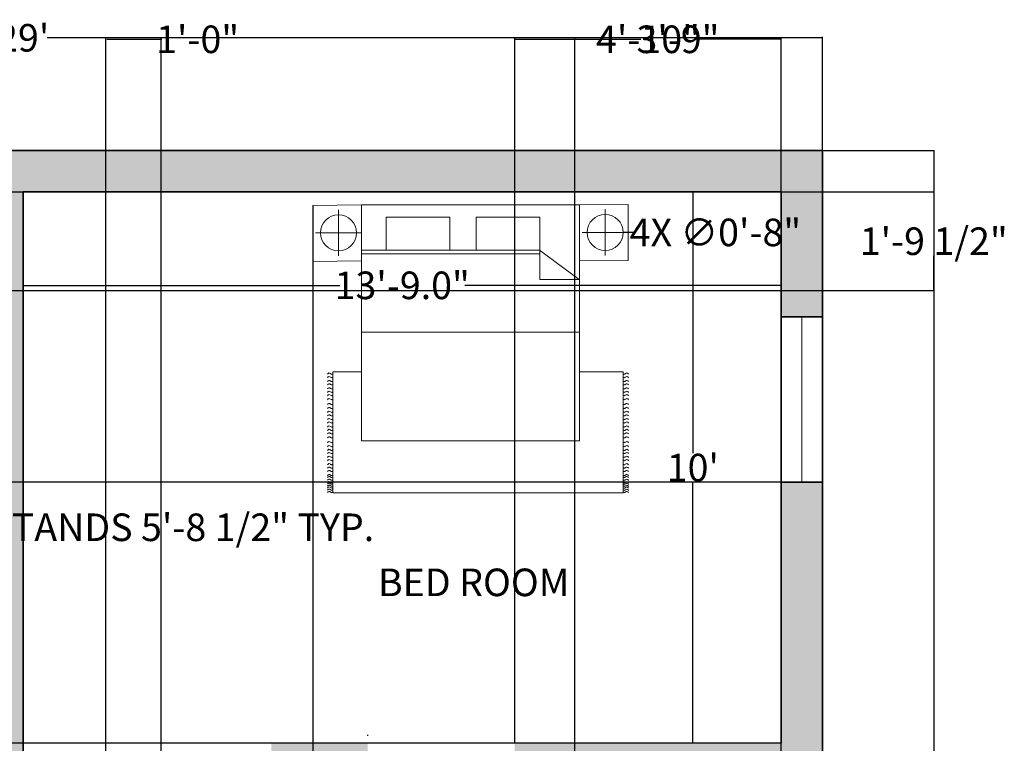
# Model space of a CAD drawing. Units: inches. Extents: x 1174 to 1615, y 3112 to 3628.
# Tile 6 of 6: x 1390 to 1604, y 3466 to 3623. Entities that reach past the tile are written whole.
import ezdxf

# ---------------------------------------------------------------- set-up
doc = ezdxf.new("R2010")
doc.units = ezdxf.units.IN
doc.header["$MEASUREMENT"] = 0
doc.layers.get('0').update_dxf_attribs({"color": 250})
for name, color, linetype, lineweight in [('A-ANNO-DIMS', 2, 'Continuous', 18), ('A-AREA-IDEN', 7, 'Continuous', 25), ('A-FURN', 8, 'Continuous', 13), ('A-GLAZ', 4, 'Continuous', 18), ('A-WALL', 7, 'Continuous', 35)]:
    doc.layers.add(name, color=color, linetype=linetype, lineweight=lineweight)
doc.layers.add('A-WALL-PATT', color=18, linetype='Continuous', lineweight=13, true_color=0x000000)
doc.styles.get("Standard").update_dxf_attribs({"font": 'arial.ttf'})
doc.dimstyles.get("Standard").update_dxf_attribs({"dimtxt": 6, "dimasz": 0.18, "dimexe": 0.18, "dimexo": 0.0625, "dimgap": 0.09, "dimtad": 0, "dimtih": 1, "dimtoh": 1, "dimdec": 1, "dimzin": 0, "dimdsep": 46, "dimlunit": 3, "dimtxsty": 'Standard', "dimcen": 0.09, "dimadec": 0, "dimazin": 0, "dimtfac": 1, "dimtdec": 1, "dimtofl": 0, "dimtmove": 0, "dimatfit": 3, "dimfxl": 1, "dimtolj": 1, "dimtzin": 0, "dimarcsym": 0})

# ---------------------------------------------------------------- blocks, each defined once
blk = doc.blocks.new('*D3')
at = {"layer": 'A-ANNO-DIMS', "color": 0, "lineweight": -2, "transparency": 16777216}
for p, q in [((1216.66, 3595.09), (1216.66, 3619.74)), ((1216.84, 3619.56), (1385.43, 3619.56)), ((1564.48, 3619.56), (1395.9, 3619.56)), ((1564.66, 3595.09), (1564.66, 3619.74))]:
    blk.add_line(p, q, dxfattribs=at)
at = {"layer": 'A-ANNO-DIMS', "color": 0, "transparency": 16777216}
for points in [[(1216.84, 3619.59), (1216.84, 3619.53), (1216.66, 3619.56)], [(1564.48, 3619.59), (1564.48, 3619.53), (1564.66, 3619.56)]]:
    blk.add_solid(points, dxfattribs=at)
at = {"layer": 'Defpoints', "color": 0, "transparency": 16777216}
for p in [(1564.66, 3619.56), (1216.66, 3595.03), (1564.66, 3595.03)]:
    blk.add_point(p, dxfattribs=at)
at = {"layer": 'A-ANNO-DIMS', "color": 0, "transparency": 16777216, "insert": (1390.66, 3619.56), "char_height": 6, "attachment_point": 5}
blk.add_mtext("\\A1;29'", dxfattribs=at)
blk = doc.blocks.new('*D15')
at = {"layer": 'A-ANNO-DIMS', "color": 0, "lineweight": -2, "transparency": 16777216}
for p, q in [((1555.6, 3586.03), (1536.24, 3586.03)), ((1536.42, 3585.85), (1536.42, 3529.18)), ((1536.42, 3466.21), (1536.42, 3522.88)), ((1555.6, 3466.03), (1536.24, 3466.03))]:
    blk.add_line(p, q, dxfattribs=at)
at = {"layer": 'A-ANNO-DIMS', "color": 0, "transparency": 16777216}
for points in [[(1536.39, 3585.85), (1536.45, 3585.85), (1536.42, 3586.03)], [(1536.39, 3466.21), (1536.45, 3466.21), (1536.42, 3466.03)]]:
    blk.add_solid(points, dxfattribs=at)
at = {"layer": 'Defpoints', "color": 0, "transparency": 16777216}
for p in [(1555.66, 3586.03), (1536.42, 3466.03), (1555.66, 3466.03)]:
    blk.add_point(p, dxfattribs=at)
at = {"layer": 'A-ANNO-DIMS', "color": 0, "transparency": 16777216, "insert": (1536.42, 3526.03), "char_height": 6, "attachment_point": 5}
blk.add_mtext("\\A1;10'", dxfattribs=at)
blk = doc.blocks.new('*D16')
at = {"layer": 'A-ANNO-DIMS', "color": 0, "lineweight": -2, "transparency": 16777216}
for p, q in [((1390.66, 3585.97), (1390.66, 3565.51)), ((1555.66, 3585.97), (1555.66, 3565.51)), ((1390.84, 3565.69), (1459.55, 3565.69)), ((1555.48, 3565.69), (1486.77, 3565.69))]:
    blk.add_line(p, q, dxfattribs=at)
at = {"layer": 'A-ANNO-DIMS', "color": 0, "transparency": 16777216}
for points in [[(1390.84, 3565.72), (1390.84, 3565.66), (1390.66, 3565.69)], [(1555.48, 3565.72), (1555.48, 3565.66), (1555.66, 3565.69)]]:
    blk.add_solid(points, dxfattribs=at)
at = {"layer": 'Defpoints', "color": 0, "transparency": 16777216}
for p in [(1390.66, 3586.03), (1555.66, 3586.03), (1555.66, 3565.69)]:
    blk.add_point(p, dxfattribs=at)
at = {"layer": 'A-ANNO-DIMS', "color": 0, "transparency": 16777216, "insert": (1473.16, 3565.69), "char_height": 6, "attachment_point": 5}
blk.add_mtext('\\A1;13\'-9.0"', dxfattribs=at)
blk = doc.blocks.new('BED-DOUBLE-WITH-NIGHTSTANDS')
for p, q in [((5.6, 61.61), (5.6, 51.56)), ((63.65, 61.72), (63.65, 51.66)), ((10.63, 56.59), (0.57, 56.59)), ((68.68, 56.69), (58.62, 56.69)), ((49.39, 52.82), (10.63, 52.82)), ((49.44, 52), (10.63, 52)), ((49.39, 52.82), (58, 46.47)), ((49.44, 52.82), (49.44, 46.47)), ((49.44, 46.47), (58, 46.47)), ((58.05, 34.96), (10.63, 34.96)), ((4.35, 0), (4.35, 26.37)), ((4.35, 26.37), (10.65, 26.37)), ((58.05, 26.37), (67.59, 26.37)), ((67.59, 26.37), (67.59, 0)), ((67.59, 0), (4.35, 0))]:
    blk.add_line(p, q)
for points in [[(0, 50.39), (10.63, 50.5), (10.63, 62.68), (0, 62.58)], [(58.05, 62.68), (58.05, 11.36), (10.63, 11.36), (10.63, 62.68)], [(58.05, 50.5), (68.68, 50.6), (68.68, 62.78), (58.05, 62.68)], [(29.88, 59.98), (29.88, 52.82), (15.98, 52.82), (15.98, 59.98)], [(49.44, 59.98), (49.44, 52.82), (35.55, 52.82), (35.55, 59.98)]]:
    blk.add_lwpolyline(points, close=True)
for centre in [(5.6, 56.59), (63.65, 56.69)]:
    blk.add_circle(centre, 3.92)
for points, knots in [([(3.23, 25.83), (3.32, 25.96), (3.52, 26.2), (3.86, 25.96), (4.14, 25.78), (4.29, 25.89), (4.35, 25.94)], [0, 0, 0, 0, 0.400747, 0.791423, 1.067667, 1.29709, 1.29709, 1.29709, 1.29709]), ([(68.71, 25.83), (68.61, 25.96), (68.42, 26.2), (68.08, 25.96), (67.8, 25.78), (67.65, 25.89), (67.58, 25.94)], [0, 0, 0, 0, 0.400747, 0.791423, 1.067667, 1.29709, 1.29709, 1.29709, 1.29709]), ([(3.23, 25.06), (3.32, 25.18), (3.52, 25.42), (3.86, 25.18), (4.14, 25.01), (4.29, 25.11), (4.35, 25.16)], [0, 0, 0, 0, 0.400747, 0.791423, 1.067667, 1.29709, 1.29709, 1.29709, 1.29709]), ([(3.23, 24.24), (3.32, 24.36), (3.52, 24.6), (3.86, 24.36), (4.14, 24.19), (4.29, 24.3), (4.35, 24.34)], [0, 0, 0, 0, 0.400747, 0.791423, 1.067667, 1.29709, 1.29709, 1.29709, 1.29709]), ([(3.23, 23.51), (3.32, 23.63), (3.52, 23.87), (3.86, 23.63), (4.14, 23.46), (4.29, 23.57), (4.35, 23.62)], [0, 0, 0, 0, 0.400747, 0.791423, 1.067667, 1.29709, 1.29709, 1.29709, 1.29709]), ([(68.71, 25.06), (68.61, 25.18), (68.42, 25.42), (68.08, 25.18), (67.8, 25.01), (67.65, 25.11), (67.58, 25.16)], [0, 0, 0, 0, 0.400747, 0.791423, 1.067667, 1.29709, 1.29709, 1.29709, 1.29709]), ([(68.71, 24.24), (68.61, 24.36), (68.42, 24.6), (68.08, 24.36), (67.8, 24.19), (67.65, 24.3), (67.58, 24.34)], [0, 0, 0, 0, 0.400747, 0.791423, 1.067667, 1.29709, 1.29709, 1.29709, 1.29709]), ([(68.71, 23.51), (68.61, 23.63), (68.42, 23.87), (68.08, 23.63), (67.8, 23.46), (67.65, 23.57), (67.58, 23.62)], [0, 0, 0, 0, 0.400747, 0.791423, 1.067667, 1.29709, 1.29709, 1.29709, 1.29709]), ([(3.23, 22.63), (3.32, 22.75), (3.52, 22.99), (3.86, 22.75), (4.14, 22.58), (4.29, 22.69), (4.35, 22.73)], [0, 0, 0, 0, 0.400747, 0.791423, 1.067667, 1.29709, 1.29709, 1.29709, 1.29709]), ([(3.23, 21.88), (3.32, 22), (3.52, 22.24), (3.86, 22), (4.14, 21.83), (4.29, 21.93), (4.35, 21.98)], [0, 0, 0, 0, 0.400747, 0.791423, 1.067667, 1.29709, 1.29709, 1.29709, 1.29709]), ([(68.71, 22.63), (68.61, 22.75), (68.42, 22.99), (68.08, 22.75), (67.8, 22.58), (67.65, 22.69), (67.58, 22.73)], [0, 0, 0, 0, 0.400747, 0.791423, 1.067667, 1.29709, 1.29709, 1.29709, 1.29709]), ([(68.71, 21.88), (68.61, 22), (68.42, 22.24), (68.08, 22), (67.8, 21.83), (67.65, 21.93), (67.58, 21.98)], [0, 0, 0, 0, 0.400747, 0.791423, 1.067667, 1.29709, 1.29709, 1.29709, 1.29709]), ([(3.23, 21.15), (3.32, 21.27), (3.52, 21.51), (3.86, 21.27), (4.14, 21.1), (4.29, 21.21), (4.35, 21.25)], [0, 0, 0, 0, 0.400747, 0.791423, 1.067667, 1.29709, 1.29709, 1.29709, 1.29709]), ([(3.23, 20.27), (3.32, 20.39), (3.52, 20.63), (3.86, 20.39), (4.14, 20.22), (4.29, 20.32), (4.35, 20.37)], [0, 0, 0, 0, 0.400747, 0.791423, 1.067667, 1.29709, 1.29709, 1.29709, 1.29709]), ([(3.23, 19.23), (3.32, 19.35), (3.52, 19.59), (3.86, 19.35), (4.14, 19.18), (4.29, 19.29), (4.35, 19.33)], [0, 0, 0, 0, 0.400747, 0.791423, 1.067667, 1.29709, 1.29709, 1.29709, 1.29709]), ([(68.71, 21.15), (68.61, 21.27), (68.42, 21.51), (68.08, 21.27), (67.8, 21.1), (67.65, 21.21), (67.58, 21.25)], [0, 0, 0, 0, 0.400747, 0.791423, 1.067667, 1.29709, 1.29709, 1.29709, 1.29709]), ([(68.71, 20.27), (68.61, 20.39), (68.42, 20.63), (68.08, 20.39), (67.8, 20.22), (67.65, 20.32), (67.58, 20.37)], [0, 0, 0, 0, 0.400747, 0.791423, 1.067667, 1.29709, 1.29709, 1.29709, 1.29709]), ([(68.71, 19.23), (68.61, 19.35), (68.42, 19.59), (68.08, 19.35), (67.8, 19.18), (67.65, 19.29), (67.58, 19.33)], [0, 0, 0, 0, 0.400747, 0.791423, 1.067667, 1.29709, 1.29709, 1.29709, 1.29709]), ([(3.23, 18.35), (3.32, 18.47), (3.52, 18.71), (3.86, 18.47), (4.14, 18.3), (4.29, 18.4), (4.35, 18.45)], [0, 0, 0, 0, 0.400747, 0.791423, 1.067667, 1.29709, 1.29709, 1.29709, 1.29709]), ([(3.23, 17.53), (3.32, 17.65), (3.52, 17.89), (3.86, 17.65), (4.14, 17.48), (4.29, 17.59), (4.35, 17.64)], [0, 0, 0, 0, 0.400747, 0.791423, 1.067667, 1.29709, 1.29709, 1.29709, 1.29709]), ([(68.71, 18.35), (68.61, 18.47), (68.42, 18.71), (68.08, 18.47), (67.8, 18.3), (67.65, 18.4), (67.58, 18.45)], [0, 0, 0, 0, 0.400747, 0.791423, 1.067667, 1.29709, 1.29709, 1.29709, 1.29709]), ([(68.71, 17.53), (68.61, 17.65), (68.42, 17.89), (68.08, 17.65), (67.8, 17.48), (67.65, 17.59), (67.58, 17.64)], [0, 0, 0, 0, 0.400747, 0.791423, 1.067667, 1.29709, 1.29709, 1.29709, 1.29709]), ([(3.23, 16.76), (3.32, 16.88), (3.52, 17.12), (3.86, 16.88), (4.14, 16.7), (4.29, 16.81), (4.35, 16.86)], [0, 0, 0, 0, 0.400747, 0.791423, 1.067667, 1.29709, 1.29709, 1.29709, 1.29709]), ([(3.23, 15.94), (3.32, 16.06), (3.52, 16.3), (3.86, 16.06), (4.14, 15.89), (4.29, 15.99), (4.35, 16.04)], [0, 0, 0, 0, 0.400747, 0.791423, 1.067667, 1.29709, 1.29709, 1.29709, 1.29709]), ([(3.23, 15.21), (3.32, 15.33), (3.52, 15.57), (3.86, 15.33), (4.14, 15.16), (4.29, 15.27), (4.35, 15.32)], [0, 0, 0, 0, 0.400747, 0.791423, 1.067667, 1.29709, 1.29709, 1.29709, 1.29709]), ([(68.71, 16.76), (68.61, 16.88), (68.42, 17.12), (68.08, 16.88), (67.8, 16.7), (67.65, 16.81), (67.58, 16.86)], [0, 0, 0, 0, 0.400747, 0.791423, 1.067667, 1.29709, 1.29709, 1.29709, 1.29709]), ([(68.71, 15.94), (68.61, 16.06), (68.42, 16.3), (68.08, 16.06), (67.8, 15.89), (67.65, 15.99), (67.58, 16.04)], [0, 0, 0, 0, 0.400747, 0.791423, 1.067667, 1.29709, 1.29709, 1.29709, 1.29709]), ([(68.71, 15.21), (68.61, 15.33), (68.42, 15.57), (68.08, 15.33), (67.8, 15.16), (67.65, 15.27), (67.58, 15.32)], [0, 0, 0, 0, 0.400747, 0.791423, 1.067667, 1.29709, 1.29709, 1.29709, 1.29709]), ([(3.23, 14.33), (3.32, 14.45), (3.52, 14.69), (3.86, 14.45), (4.14, 14.28), (4.29, 14.38), (4.35, 14.43)], [0, 0, 0, 0, 0.400747, 0.791423, 1.067667, 1.29709, 1.29709, 1.29709, 1.29709]), ([(3.23, 13.58), (3.32, 13.7), (3.52, 13.94), (3.86, 13.7), (4.14, 13.53), (4.29, 13.63), (4.35, 13.68)], [0, 0, 0, 0, 0.400747, 0.791423, 1.067667, 1.29709, 1.29709, 1.29709, 1.29709]), ([(3.23, 12.85), (3.32, 12.97), (3.52, 13.21), (3.86, 12.97), (4.14, 12.8), (4.29, 12.9), (4.35, 12.95)], [0, 0, 0, 0, 0.400747, 0.791423, 1.067667, 1.29709, 1.29709, 1.29709, 1.29709]), ([(68.71, 14.33), (68.61, 14.45), (68.42, 14.69), (68.08, 14.45), (67.8, 14.28), (67.65, 14.38), (67.58, 14.43)], [0, 0, 0, 0, 0.400747, 0.791423, 1.067667, 1.29709, 1.29709, 1.29709, 1.29709]), ([(68.71, 13.58), (68.61, 13.7), (68.42, 13.94), (68.08, 13.7), (67.8, 13.53), (67.65, 13.63), (67.58, 13.68)], [0, 0, 0, 0, 0.400747, 0.791423, 1.067667, 1.29709, 1.29709, 1.29709, 1.29709]), ([(68.71, 12.85), (68.61, 12.97), (68.42, 13.21), (68.08, 12.97), (67.8, 12.8), (67.65, 12.9), (67.58, 12.95)], [0, 0, 0, 0, 0.400747, 0.791423, 1.067667, 1.29709, 1.29709, 1.29709, 1.29709]), ([(3.23, 11.97), (3.32, 12.09), (3.52, 12.33), (3.86, 12.09), (4.14, 11.92), (4.29, 12.02), (4.35, 12.07)], [0, 0, 0, 0, 0.400747, 0.791423, 1.067667, 1.29709, 1.29709, 1.29709, 1.29709]), ([(3.23, 10.93), (3.32, 11.05), (3.52, 11.29), (3.86, 11.05), (4.14, 10.88), (4.29, 10.99), (4.35, 11.03)], [0, 0, 0, 0, 0.400747, 0.791423, 1.067667, 1.29709, 1.29709, 1.29709, 1.29709]), ([(68.71, 11.97), (68.61, 12.09), (68.42, 12.33), (68.08, 12.09), (67.8, 11.92), (67.65, 12.02), (67.58, 12.07)], [0, 0, 0, 0, 0.400747, 0.791423, 1.067667, 1.29709, 1.29709, 1.29709, 1.29709]), ([(68.71, 10.93), (68.61, 11.05), (68.42, 11.29), (68.08, 11.05), (67.8, 10.88), (67.65, 10.99), (67.58, 11.03)], [0, 0, 0, 0, 0.400747, 0.791423, 1.067667, 1.29709, 1.29709, 1.29709, 1.29709]), ([(3.23, 10.05), (3.32, 10.17), (3.52, 10.41), (3.86, 10.17), (4.14, 10), (4.29, 10.1), (4.35, 10.15)], [0, 0, 0, 0, 0.400747, 0.791423, 1.067667, 1.29709, 1.29709, 1.29709, 1.29709]), ([(3.23, 9.23), (3.32, 9.35), (3.52, 9.59), (3.86, 9.35), (4.14, 9.18), (4.29, 9.29), (4.35, 9.34)], [0, 0, 0, 0, 0.400747, 0.791423, 1.067667, 1.29709, 1.29709, 1.29709, 1.29709]), ([(3.23, 8.54), (3.32, 8.66), (3.52, 8.9), (3.86, 8.66), (4.14, 8.49), (4.29, 8.6), (4.35, 8.65)], [0, 0, 0, 0, 0.400747, 0.791423, 1.067667, 1.29709, 1.29709, 1.29709, 1.29709]), ([(68.71, 10.05), (68.61, 10.17), (68.42, 10.41), (68.08, 10.17), (67.8, 10), (67.65, 10.1), (67.58, 10.15)], [0, 0, 0, 0, 0.400747, 0.791423, 1.067667, 1.29709, 1.29709, 1.29709, 1.29709]), ([(68.71, 9.23), (68.61, 9.35), (68.42, 9.59), (68.08, 9.35), (67.8, 9.18), (67.65, 9.29), (67.58, 9.34)], [0, 0, 0, 0, 0.400747, 0.791423, 1.067667, 1.29709, 1.29709, 1.29709, 1.29709]), ([(68.71, 8.54), (68.61, 8.66), (68.42, 8.9), (68.08, 8.66), (67.8, 8.49), (67.65, 8.6), (67.58, 8.65)], [0, 0, 0, 0, 0.400747, 0.791423, 1.067667, 1.29709, 1.29709, 1.29709, 1.29709]), ([(3.23, 7.73), (3.32, 7.85), (3.52, 8.09), (3.86, 7.85), (4.14, 7.68), (4.29, 7.78), (4.35, 7.83)], [0, 0, 0, 0, 0.400747, 0.791423, 1.067667, 1.29709, 1.29709, 1.29709, 1.29709]), ([(3.23, 7), (3.32, 7.12), (3.52, 7.36), (3.86, 7.12), (4.14, 6.95), (4.29, 7.05), (4.35, 7.1)], [0, 0, 0, 0, 0.400747, 0.791423, 1.067667, 1.29709, 1.29709, 1.29709, 1.29709]), ([(68.71, 7.73), (68.61, 7.85), (68.42, 8.09), (68.08, 7.85), (67.8, 7.68), (67.65, 7.78), (67.58, 7.83)], [0, 0, 0, 0, 0.400747, 0.791423, 1.067667, 1.29709, 1.29709, 1.29709, 1.29709]), ([(68.71, 7), (68.61, 7.12), (68.42, 7.36), (68.08, 7.12), (67.8, 6.95), (67.65, 7.05), (67.58, 7.1)], [0, 0, 0, 0, 0.400747, 0.791423, 1.067667, 1.29709, 1.29709, 1.29709, 1.29709]), ([(3.23, 6.12), (3.32, 6.24), (3.52, 6.48), (3.86, 6.24), (4.14, 6.06), (4.29, 6.17), (4.35, 6.22)], [0, 0, 0, 0, 0.400747, 0.791423, 1.067667, 1.29709, 1.29709, 1.29709, 1.29709]), ([(3.23, 5.36), (3.32, 5.49), (3.52, 5.73), (3.86, 5.49), (4.14, 5.31), (4.29, 5.42), (4.35, 5.47)], [0, 0, 0, 0, 0.400747, 0.791423, 1.067667, 1.29709, 1.29709, 1.29709, 1.29709]), ([(3.23, 4.64), (3.32, 4.76), (3.52, 5), (3.86, 4.76), (4.14, 4.58), (4.29, 4.69), (4.35, 4.74)], [0, 0, 0, 0, 0.400747, 0.791423, 1.067667, 1.29709, 1.29709, 1.29709, 1.29709]), ([(68.71, 6.12), (68.61, 6.24), (68.42, 6.48), (68.08, 6.24), (67.8, 6.06), (67.65, 6.17), (67.58, 6.22)], [0, 0, 0, 0, 0.400747, 0.791423, 1.067667, 1.29709, 1.29709, 1.29709, 1.29709]), ([(68.71, 5.36), (68.61, 5.49), (68.42, 5.73), (68.08, 5.49), (67.8, 5.31), (67.65, 5.42), (67.58, 5.47)], [0, 0, 0, 0, 0.400747, 0.791423, 1.067667, 1.29709, 1.29709, 1.29709, 1.29709]), ([(68.71, 4.64), (68.61, 4.76), (68.42, 5), (68.08, 4.76), (67.8, 4.59), (67.66, 4.69), (67.59, 4.73)], [0, 0, 0, 0, 0.400747, 0.791423, 1.067667, 1.283686, 1.283686, 1.283686, 1.283686]), ([(3.23, 3.75), (3.32, 3.88), (3.52, 4.11), (3.86, 3.88), (4.14, 3.7), (4.29, 3.81), (4.35, 3.86)], [0, 0, 0, 0, 0.400747, 0.791423, 1.067667, 1.29709, 1.29709, 1.29709, 1.29709]), ([(3.23, 3.32), (3.32, 3.45), (3.51, 3.7), (3.86, 3.44), (4.14, 3.27), (4.29, 3.38), (4.35, 3.43)], [0, 0, 0, 0, 0.407265, 0.802015, 1.07826, 1.307683, 1.307683, 1.307683, 1.307683]), ([(3.23, 2.76), (3.32, 2.88), (3.52, 3.12), (3.86, 2.88), (4.14, 2.71), (4.29, 2.81), (4.35, 2.86)], [0, 0, 0, 0, 0.400747, 0.791423, 1.067667, 1.29709, 1.29709, 1.29709, 1.29709]), ([(3.23, 2.18), (3.32, 2.31), (3.52, 2.55), (3.86, 2.31), (4.14, 2.13), (4.29, 2.24), (4.35, 2.29)], [0, 0, 0, 0, 0.400747, 0.791423, 1.067667, 1.29709, 1.29709, 1.29709, 1.29709]), ([(3.23, 1.88), (3.32, 2), (3.52, 2.24), (3.86, 2), (4.14, 1.82), (4.29, 1.93), (4.35, 1.98)], [0, 0, 0, 0, 0.400747, 0.791423, 1.067667, 1.29709, 1.29709, 1.29709, 1.29709]), ([(68.71, 3.75), (68.61, 3.88), (68.42, 4.11), (68.08, 3.88), (67.8, 3.7), (67.66, 3.8), (67.59, 3.85)], [0, 0, 0, 0, 0.400747, 0.791423, 1.067667, 1.283686, 1.283686, 1.283686, 1.283686]), ([(68.71, 3.32), (68.61, 3.45), (68.42, 3.69), (68.08, 3.45), (67.8, 3.27), (67.66, 3.38), (67.59, 3.42)], [0, 0, 0, 0, 0.402903, 0.794912, 1.071156, 1.287177, 1.287177, 1.287177, 1.287177]), ([(68.71, 2.73), (68.61, 2.85), (68.42, 3.09), (68.08, 2.85), (67.8, 2.68), (67.66, 2.78), (67.59, 2.82)], [0, 0, 0, 0, 0.400747, 0.791423, 1.067667, 1.283686, 1.283686, 1.283686, 1.283686]), ([(68.71, 2.16), (68.61, 2.28), (68.42, 2.52), (68.08, 2.28), (67.8, 2.11), (67.66, 2.21), (67.59, 2.25)], [0, 0, 0, 0, 0.400747, 0.791423, 1.067667, 1.283686, 1.283686, 1.283686, 1.283686]), ([(3.23, 1.46), (3.32, 1.58), (3.52, 1.82), (3.86, 1.58), (4.14, 1.4), (4.29, 1.51), (4.35, 1.56)], [0, 0, 0, 0, 0.400747, 0.791423, 1.067667, 1.29709, 1.29709, 1.29709, 1.29709]), ([(3.23, 1.06), (3.32, 1.18), (3.52, 1.42), (3.86, 1.18), (4.14, 1.01), (4.29, 1.11), (4.35, 1.16)], [0, 0, 0, 0, 0.400747, 0.791423, 1.067667, 1.29709, 1.29709, 1.29709, 1.29709]), ([(3.23, 0.57), (3.32, 0.7), (3.52, 0.93), (3.86, 0.7), (4.14, 0.52), (4.29, 0.63), (4.35, 0.68)], [0, 0, 0, 0, 0.400747, 0.791423, 1.067667, 1.29709, 1.29709, 1.29709, 1.29709]), ([(3.23, 0.07), (3.32, 0.19), (3.52, 0.43), (3.86, 0.19), (4.14, 0.02), (4.29, 0.13), (4.35, 0.18)], [0, 0, 0, 0, 0.400747, 0.791423, 1.067667, 1.29709, 1.29709, 1.29709, 1.29709]), ([(68.71, 1.43), (68.61, 1.55), (68.42, 1.79), (68.08, 1.55), (67.8, 1.38), (67.65, 1.48), (67.58, 1.53)], [0, 0, 0, 0, 0.400747, 0.791423, 1.067667, 1.29709, 1.29709, 1.29709, 1.29709]), ([(68.71, 1.03), (68.61, 1.15), (68.42, 1.39), (68.08, 1.15), (67.8, 0.98), (67.65, 1.09), (67.58, 1.13)], [0, 0, 0, 0, 0.400747, 0.791423, 1.067667, 1.29709, 1.29709, 1.29709, 1.29709]), ([(68.71, 0.55), (68.61, 0.67), (68.42, 0.91), (68.08, 0.67), (67.8, 0.49), (67.65, 0.6), (67.58, 0.65)], [0, 0, 0, 0, 0.400747, 0.791423, 1.067667, 1.29709, 1.29709, 1.29709, 1.29709]), ([(68.71, 0.07), (68.61, 0.19), (68.42, 0.43), (68.08, 0.19), (67.8, 0.02), (67.65, 0.13), (67.58, 0.18)], [0, 0, 0, 0, 0.400747, 0.791423, 1.067667, 1.29709, 1.29709, 1.29709, 1.29709]), ([(68.71, 1.85), (68.61, 1.97), (68.42, 2.21), (68.08, 1.97), (67.8, 1.8), (67.66, 1.9), (67.59, 1.94)], [0, 0, 0, 0, 0.400747, 0.791423, 1.067667, 1.283686, 1.283686, 1.283686, 1.283686])]:
    blk.add_open_spline(points, degree=3, knots=knots)
blk = doc.blocks.new('WINDOW-36IN')
for p, q in [((-4.5, -36), (-4.5, 0)), ((0, 0), (0, -36)), ((4.5, 0), (4.5, -36))]:
    blk.add_line(p, q)
blk = doc.blocks.new('*D30')
at = {"layer": 'A-ANNO-DIMS', "color": 0, "lineweight": -2, "transparency": 16777216}
for p, q in [((1261.16, 3523.29), (1261.16, 3512.86)), ((1329.87, 3523.29), (1329.87, 3512.86)), ((1261.34, 3513.04), (1329.69, 3513.04)), ((1329.87, 3513.04), (1330.05, 3513.04))]:
    blk.add_line(p, q, dxfattribs=at)
at = {"layer": 'A-ANNO-DIMS', "color": 0, "transparency": 16777216}
for points in [[(1261.34, 3513.07), (1261.34, 3513.01), (1261.16, 3513.04)], [(1329.69, 3513.07), (1329.69, 3513.01), (1329.87, 3513.04)]]:
    blk.add_solid(points, dxfattribs=at)
at = {"layer": 'Defpoints', "color": 0, "transparency": 16777216}
for p in [(1261.16, 3523.35), (1329.87, 3523.35), (1329.87, 3513.04)]:
    blk.add_point(p, dxfattribs=at)
at = {"layer": 'A-ANNO-DIMS', "color": 0, "transparency": 16777216, "insert": (1400.23, 3513.04), "char_height": 6, "attachment_point": 5}
blk.add_mtext('\\A1;BED & NIGHTSTANDS 5\'-8 1/2" TYP.', dxfattribs=at)
blk = doc.blocks.new('*D41')
at = {"layer": 'A-ANNO-DIMS', "color": 0, "lineweight": -2, "transparency": 16777216}
for p, q in [((1564.73, 3595.03), (1589.04, 3595.03)), ((1588.86, 3594.85), (1588.86, 3373.18)), ((1588.86, 3145.21), (1588.86, 3366.87)), ((1439.51, 3145.03), (1589.04, 3145.03))]:
    blk.add_line(p, q, dxfattribs=at)
at = {"layer": 'A-ANNO-DIMS', "color": 0, "transparency": 16777216}
for points in [[(1588.83, 3594.85), (1588.89, 3594.85), (1588.86, 3595.03)], [(1588.83, 3145.21), (1588.89, 3145.21), (1588.86, 3145.03)]]:
    blk.add_solid(points, dxfattribs=at)
at = {"layer": 'Defpoints', "color": 0, "transparency": 16777216}
for p in [(1564.66, 3595.03), (1588.86, 3595.03), (1439.45, 3145.03)]:
    blk.add_point(p, dxfattribs=at)
at = {"layer": 'A-ANNO-DIMS', "color": 0, "transparency": 16777216, "insert": (1588.86, 3370.03), "char_height": 6, "attachment_point": 5}
blk.add_mtext('\\A1;37\'-6"', dxfattribs=at)
blk = doc.blocks.new('*D47')
at = {"layer": 'A-ANNO-DIMS', "color": 0, "lineweight": -2, "transparency": 16777216}
for p, q in [((1225.73, 3586.03), (1589.04, 3586.03)), ((1588.86, 3585.85), (1588.86, 3578.48)), ((1588.86, 3564.73), (1588.86, 3572.1)), ((1225.73, 3564.55), (1589.04, 3564.55))]:
    blk.add_line(p, q, dxfattribs=at)
at = {"layer": 'A-ANNO-DIMS', "color": 0, "transparency": 16777216}
for points in [[(1588.83, 3585.85), (1588.89, 3585.85), (1588.86, 3586.03)], [(1588.83, 3564.73), (1588.89, 3564.73), (1588.86, 3564.55)]]:
    blk.add_solid(points, dxfattribs=at)
at = {"layer": 'Defpoints', "color": 0, "transparency": 16777216}
for p in [(1225.66, 3586.03), (1225.66, 3564.55), (1588.86, 3564.55)]:
    blk.add_point(p, dxfattribs=at)
at = {"layer": 'A-ANNO-DIMS', "color": 0, "transparency": 16777216, "insert": (1588.86, 3575.29), "char_height": 6, "attachment_point": 5}
blk.add_mtext('\\A1;1\'-9 1/2"', dxfattribs=at)
blk = doc.blocks.new('*D50')
at = {"layer": 'A-ANNO-DIMS', "color": 0, "lineweight": -2, "transparency": 16777216}
for p, q in [((1555.6, 3522.83), (1192.28, 3522.83)), ((1192.46, 3522.65), (1192.46, 3497.58)), ((1192.46, 3466.21), (1192.46, 3491.28)), ((1555.6, 3466.03), (1192.28, 3466.03))]:
    blk.add_line(p, q, dxfattribs=at)
at = {"layer": 'A-ANNO-DIMS', "color": 0, "transparency": 16777216}
for points in [[(1192.43, 3522.65), (1192.49, 3522.65), (1192.46, 3522.83)], [(1192.43, 3466.21), (1192.49, 3466.21), (1192.46, 3466.03)]]:
    blk.add_solid(points, dxfattribs=at)
at = {"layer": 'Defpoints', "color": 0, "transparency": 16777216}
for p in [(1555.66, 3522.83), (1192.46, 3466.03), (1555.66, 3466.03)]:
    blk.add_point(p, dxfattribs=at)
at = {"layer": 'A-ANNO-DIMS', "color": 0, "transparency": 16777216, "insert": (1192.46, 3494.43), "char_height": 6, "attachment_point": 5}
blk.add_mtext('\\A1;4\'-9"', dxfattribs=at)
blk = doc.blocks.new('*D55')
at = {"layer": 'A-ANNO-DIMS', "color": 0, "lineweight": -2, "transparency": 16777216}
for p, q in [((1497.66, 3466.09), (1497.66, 3619.41)), ((1497.84, 3619.23), (1516.15, 3619.23)), ((1555.48, 3619.23), (1537.18, 3619.23)), ((1555.66, 3466.09), (1555.66, 3619.41))]:
    blk.add_line(p, q, dxfattribs=at)
at = {"layer": 'A-ANNO-DIMS', "color": 0, "transparency": 16777216}
for points in [[(1497.84, 3619.26), (1497.84, 3619.2), (1497.66, 3619.23)], [(1555.48, 3619.26), (1555.48, 3619.2), (1555.66, 3619.23)]]:
    blk.add_solid(points, dxfattribs=at)
at = {"layer": 'Defpoints', "color": 0, "transparency": 16777216}
for p in [(1555.66, 3619.23), (1497.66, 3466.03), (1555.66, 3466.03)]:
    blk.add_point(p, dxfattribs=at)
at = {"layer": 'A-ANNO-DIMS', "color": 0, "transparency": 16777216, "insert": (1526.66, 3619.23), "char_height": 6, "attachment_point": 5}
blk.add_mtext('\\A1;4\'-10"', dxfattribs=at)
blk = doc.blocks.new('*D59')
at = {"layer": 'A-ANNO-DIMS', "color": 0, "lineweight": -2, "transparency": 16777216}
for p, q in [((1408.66, 3268.09), (1408.66, 3619.41)), ((1408.84, 3619.23), (1420.48, 3619.23)), ((1420.66, 3268.09), (1420.66, 3619.41)), ((1420.66, 3619.23), (1420.84, 3619.23))]:
    blk.add_line(p, q, dxfattribs=at)
at = {"layer": 'A-ANNO-DIMS', "color": 0, "transparency": 16777216}
for points in [[(1408.84, 3619.26), (1408.84, 3619.2), (1408.66, 3619.23)], [(1420.48, 3619.26), (1420.48, 3619.2), (1420.66, 3619.23)]]:
    blk.add_solid(points, dxfattribs=at)
at = {"layer": 'Defpoints', "color": 0, "transparency": 16777216}
for p in [(1420.66, 3619.23), (1408.66, 3268.03), (1420.66, 3268.03)]:
    blk.add_point(p, dxfattribs=at)
at = {"layer": 'A-ANNO-DIMS', "color": 0, "transparency": 16777216, "insert": (1428.63, 3619.23), "char_height": 6, "attachment_point": 5}
blk.add_mtext('\\A1;1\'-0"', dxfattribs=at)
blk = doc.blocks.new('*D70')
at = {"layer": 'A-ANNO-DIMS', "color": 0, "lineweight": -2, "transparency": 16777216}
for p, q in [((1390.66, 3585.97), (1390.66, 3120.65)), ((1453.68, 3583.03), (1453.68, 3120.65)), ((1390.84, 3120.83), (1414.11, 3120.83)), ((1453.5, 3120.83), (1430.24, 3120.83))]:
    blk.add_line(p, q, dxfattribs=at)
at = {"layer": 'A-ANNO-DIMS', "color": 0, "transparency": 16777216}
for points in [[(1390.84, 3120.86), (1390.84, 3120.8), (1390.66, 3120.83)], [(1453.5, 3120.86), (1453.5, 3120.8), (1453.68, 3120.83)]]:
    blk.add_solid(points, dxfattribs=at)
at = {"layer": 'Defpoints', "color": 0, "transparency": 16777216}
for p in [(1390.66, 3586.03), (1453.68, 3583.1), (1453.68, 3120.83)]:
    blk.add_point(p, dxfattribs=at)
at = {"layer": 'A-ANNO-DIMS', "color": 0, "transparency": 16777216, "insert": (1422.17, 3120.83), "char_height": 6, "attachment_point": 5}
blk.add_mtext('\\A1;5\'-3"', dxfattribs=at)
blk = doc.blocks.new('*D73')
at = {"layer": 'A-ANNO-DIMS', "color": 0, "lineweight": -2, "transparency": 16777216}
for p, q in [((1510.72, 3286.5), (1510.72, 3619.41)), ((1510.9, 3619.23), (1525.13, 3619.23)), ((1555.48, 3619.23), (1541.25, 3619.23)), ((1555.66, 3284.24), (1555.66, 3619.41))]:
    blk.add_line(p, q, dxfattribs=at)
at = {"layer": 'A-ANNO-DIMS', "color": 0, "transparency": 16777216}
for points in [[(1510.9, 3619.26), (1510.9, 3619.2), (1510.72, 3619.23)], [(1555.48, 3619.26), (1555.48, 3619.2), (1555.66, 3619.23)]]:
    blk.add_solid(points, dxfattribs=at)
at = {"layer": 'Defpoints', "color": 0, "transparency": 16777216}
for p in [(1510.72, 3619.23), (1510.72, 3286.44), (1555.66, 3284.17)]:
    blk.add_point(p, dxfattribs=at)
at = {"layer": 'A-ANNO-DIMS', "color": 0, "transparency": 16777216, "insert": (1533.19, 3619.23), "char_height": 6, "attachment_point": 5}
blk.add_mtext('\\A1;3\'-9"', dxfattribs=at)
blk = doc.blocks.new('*D77')
at = {"layer": 'A-ANNO-DIMS', "color": 0, "lineweight": -2, "transparency": 16777216}
for p, q in [((1465.66, 3467.7), (1465.66, 3467.88)), ((1465.57, 3467.79), (1465.75, 3467.79)), ((1497.19, 3423.93), (1485.47, 3440.23)), ((1497.37, 3423.93), (1497.19, 3423.93))]:
    blk.add_line(p, q, dxfattribs=at)
at = {"layer": 'A-ANNO-DIMS', "color": 0, "transparency": 16777216}
blk.add_solid([(1485.5, 3440.25), (1485.45, 3440.21), (1485.37, 3440.38)], dxfattribs=at)
at = {"layer": 'Defpoints', "color": 0, "transparency": 16777216}
for p in [(1465.66, 3467.79), (1485.37, 3440.38)]:
    blk.add_point(p, dxfattribs=at)
at = {"layer": 'A-ANNO-DIMS', "color": 0, "transparency": 16777216, "insert": (1517.08, 3423.93), "char_height": 6, "attachment_point": 5}
blk.add_mtext('\\A1;3X R2\'-10"', dxfattribs=at)
blk = doc.blocks.new('*D78')
at = {"layer": 'A-ANNO-DIMS', "color": 0, "lineweight": -2, "transparency": 16777216}
for p, q in [((1517.24, 3577.21), (1517.42, 3577.21)), ((1517.33, 3577.12), (1517.33, 3577.3)), ((1523.61, 3577.21), (1521.43, 3577.21))]:
    blk.add_line(p, q, dxfattribs=at)
at = {"layer": 'A-ANNO-DIMS', "color": 0, "transparency": 16777216}
blk.add_solid([(1521.43, 3577.24), (1521.43, 3577.18), (1521.25, 3577.21)], dxfattribs=at)
at = {"layer": 'Defpoints', "color": 0, "transparency": 16777216}
for p in [(1513.41, 3577.21), (1521.25, 3577.21)]:
    blk.add_point(p, dxfattribs=at)
at = {"layer": 'A-ANNO-DIMS', "color": 0, "transparency": 16777216, "insert": (1541.34, 3577.21), "char_height": 6, "attachment_point": 5}
blk.add_mtext('\\A1;4X ∅0\'-8"', dxfattribs=at)

msp = doc.modelspace()

# ---------------------------------------------------------------- hatches: boundary and pattern name
at = {"layer": 'A-WALL-PATT'}
h = msp.add_hatch(color=256, dxfattribs=at)
h.dxf.hatch_style = 1
h.paths.add_polyline_path([(1564.66, 3595.03), (1216.66, 3595.03), (1216.66, 3564.55), (1225.66, 3564.55), (1225.66, 3586.03), (1381.66, 3586.03), (1381.66, 3385.03), (1380.66, 3385.03), (1380.66, 3376.03), (1381.66, 3376.03), (1407.66, 3376.03), (1407.66, 3385.03), (1390.66, 3385.03), (1390.66, 3586.03), (1555.66, 3586.03), (1555.66, 3558.83), (1564.66, 3558.83)])
h.paths.add_polyline_path([(1564.66, 3408.64), (1555.66, 3408.64), (1555.66, 3385.03), (1453.66, 3385.03), (1453.66, 3457.03), (1465.66, 3457.03), (1465.66, 3466.03), (1453.66, 3466.03), (1444.66, 3466.03), (1444.66, 3385.03), (1443.66, 3385.03), (1443.66, 3376.03), (1444.66, 3376.03), (1555.66, 3376.03), (1555.66, 3320.17), (1564.66, 3320.17)])
h.paths.add_polyline_path([(1564.66, 3522.83), (1555.66, 3522.83), (1555.66, 3466.03), (1497.66, 3466.03), (1497.66, 3457.03), (1555.66, 3457.03), (1555.66, 3432.64), (1564.66, 3432.64)], flags=17)
h.paths.add_polyline_path([(1344.66, 3385.03), (1336.66, 3385.03), (1336.66, 3466.03), (1269.66, 3466.03), (1269.66, 3457.03), (1327.66, 3457.03), (1327.66, 3385.03), (1225.66, 3385.03), (1225.66, 3413.31), (1216.66, 3413.31), (1216.66, 3319.63), (1225.66, 3319.63), (1225.66, 3376.03), (1344.66, 3376.03)])
h.paths.add_polyline_path([(1237.66, 3466.03), (1225.66, 3466.03), (1225.66, 3528.55), (1216.66, 3528.55), (1216.66, 3437.31), (1225.66, 3437.31), (1225.66, 3457.03), (1237.66, 3457.03)], flags=17)
h.paths.add_polyline_path([(1265.25, 3184.03), (1225.66, 3184.03), (1225.66, 3283.63), (1216.66, 3283.63), (1216.66, 3175.03), (1265.25, 3175.03)])
h.paths.add_polyline_path([(1372.66, 3184.03), (1360.66, 3184.03), (1360.66, 3268.03), (1376.66, 3268.03), (1376.66, 3277.03), (1360.66, 3277.03), (1360.66, 3313.03), (1351.66, 3313.03), (1351.66, 3184.03), (1301.25, 3184.03), (1301.25, 3175.03), (1372.66, 3175.03)])
h.paths.add_polyline_path([(1460.02, 3184.03), (1429.66, 3184.03), (1429.66, 3277.03), (1408.66, 3277.03), (1408.66, 3268.03), (1420.66, 3268.03), (1420.66, 3184.03), (1408.66, 3184.03), (1408.66, 3175.03), (1460.02, 3175.03)])
h.paths.add_polyline_path([(1564.66, 3284.17), (1555.66, 3284.17), (1555.66, 3184.03), (1520.02, 3184.03), (1520.02, 3175.03), (1564.66, 3175.03)])

# ---------------------------------------------------------------- linework, layer by layer
at = {"layer": 'A-WALL'}
for p, q in [((1216.66, 3595.03), (1564.66, 3595.03)), ((1564.66, 3595.03), (1564.66, 3175.03)), ((1390.66, 3586.03), (1390.66, 3385.03)), ((1390.66, 3586.03), (1555.66, 3586.03)), ((1555.66, 3586.03), (1555.66, 3466.03)), ((1555.66, 3558.83), (1564.66, 3558.83)), ((1564.66, 3522.83), (1555.66, 3522.83))]:
    msp.add_line(p, q, dxfattribs=at)

# ---------------------------------------------------------------- block references
at = {"layer": 'A-FURN'}
msp.add_blockref('BED-DOUBLE-WITH-NIGHTSTANDS', (1453.68, 3520.52), dxfattribs=at)
at = {"layer": 'A-GLAZ', "rotation": 180}
msp.add_blockref('WINDOW-36IN', (1560.16, 3522.83), dxfattribs=at)

# ---------------------------------------------------------------- texts
at = {"layer": 'A-AREA-IDEN', "insert": (1467.88, 3504.05), "char_height": 6, "attachment_point": 1}
msp.add_mtext_dynamic_manual_height_columns('BED ROOM', width=75.1452, gutter_width=1, heights=[0], dxfattribs=at)

# ---------------------------------------------------------------- dimensions: what is measured, and where the dimension line sits
at = {"layer": 'A-ANNO-DIMS'}
for base, p1, p2, override, picture, middle in [((1564.66, 3619.56), (1216.66, 3595.03), (1564.66, 3595.03), {"dimclrd": 0, "dimclre": 0, "dimclrt": 0}, '*D3', (1390.66, 3619.56)), ((1420.66, 3619.23), (1408.66, 3268.03), (1420.66, 3268.03), {"dimdec": 1, "dimlfac": 1, "dimrnd": 0, "dimzin": 1, "dimdsep": 46, "dimlunit": 4, "dimfrac": 2}, '*D59', (1428.63, 3619.23)), ((1555.66, 3619.23), (1497.66, 3466.03), (1555.66, 3466.03), {"dimdec": 1, "dimlfac": 1, "dimrnd": 0, "dimzin": 1, "dimdsep": 46, "dimlunit": 4, "dimfrac": 2}, '*D55', (1526.66, 3619.23)), ((1510.72, 3619.23), (1555.66, 3284.17), (1510.72, 3286.44), {"dimdec": 1, "dimlfac": 1, "dimrnd": 0, "dimzin": 1, "dimdsep": 46, "dimlunit": 4, "dimfrac": 2}, '*D73', (1533.19, 3619.23)), ((1555.66, 3565.69), (1390.66, 3586.03), (1555.66, 3586.03), {"dimclrd": 0, "dimclre": 0, "dimclrt": 0}, '*D16', (1473.16, 3565.69)), ((1453.68, 3120.83), (1390.66, 3586.03), (1453.68, 3583.1), {"dimdec": 1, "dimlfac": 1, "dimrnd": 0, "dimzin": 1, "dimdsep": 46, "dimlunit": 4, "dimfrac": 2}, '*D70', (1422.17, 3120.83))]:
    dim = msp.add_linear_dim(base=base, p1=p1, p2=p2, dimstyle='Standard', override=override, dxfattribs=at)
    dim.commit()
    dim.dimension.update_dxf_attribs({"geometry": picture, "text_midpoint": middle})
for base, p1, p2, override, picture, middle in [((1588.86, 3595.03), (1439.45, 3145.03), (1564.66, 3595.03), {"dimdec": 1, "dimlfac": 1, "dimrnd": 0, "dimzin": 1, "dimdsep": 46, "dimlunit": 4, "dimfrac": 2}, '*D41', (1588.86, 3370.03)), ((1588.86, 3564.55), (1225.66, 3586.03), (1225.66, 3564.55), {"dimdec": 1, "dimlfac": 1, "dimrnd": 0, "dimzin": 1, "dimdsep": 46, "dimlunit": 4, "dimfrac": 2}, '*D47', (1588.86, 3575.29)), ((1536.42, 3466.03), (1555.66, 3586.03), (1555.66, 3466.03), {"dimclrd": 0, "dimclre": 0, "dimclrt": 0}, '*D15', (1536.42, 3526.03)), ((1192.46, 3466.03), (1555.66, 3522.83), (1555.66, 3466.03), {"dimdec": 1, "dimlfac": 1, "dimrnd": 0, "dimzin": 1, "dimdsep": 46, "dimlunit": 4, "dimfrac": 2}, '*D50', (1192.46, 3494.43))]:
    dim = msp.add_linear_dim(base=base, p1=p1, p2=p2, angle=90, dimstyle='Standard', override=override, dxfattribs=at)
    dim.commit()
    dim.dimension.update_dxf_attribs({"geometry": picture, "text_midpoint": middle})
dim = msp.add_diameter_dim_2p(p1=(1513.41, 3577.21), p2=(1521.25, 3577.21), text='4X <>', dimstyle='Standard', override={"dimdec": 1, "dimlfac": 1, "dimrnd": 0, "dimzin": 1, "dimdsep": 46, "dimlunit": 4, "dimfrac": 2}, dxfattribs=at)
dim.commit()
dim.dimension.update_dxf_attribs({"geometry": '*D78', "text_midpoint": (1523.61, 3577.21), "dimtype": 163})
dim = msp.add_linear_dim(base=(1329.87, 3513.04), p1=(1261.16, 3523.35), p2=(1329.87, 3523.35), text='BED & NIGHTSTANDS <> TYP.', dimstyle='Standard', override={"dimdec": 1, "dimlfac": 1, "dimrnd": 0, "dimzin": 1, "dimdsep": 46, "dimlunit": 4, "dimfrac": 2}, dxfattribs=at)
dim.commit()
dim.dimension.update_dxf_attribs({"geometry": '*D30', "text_midpoint": (1400.23, 3513.04)})
dim = msp.add_radius_dim(center=(1465.66, 3467.79), mpoint=(1485.37, 3440.38), text='3X <>', dimstyle='Standard', override={"dimdec": 1, "dimlfac": 1, "dimrnd": 0, "dimzin": 1, "dimdsep": 46, "dimlunit": 4, "dimfrac": 2}, dxfattribs=at)
dim.commit()
dim.dimension.update_dxf_attribs({"geometry": '*D77', "text_midpoint": (1517.08, 3423.93), "dimtype": 164})

doc.saveas('drawing.dxf')
